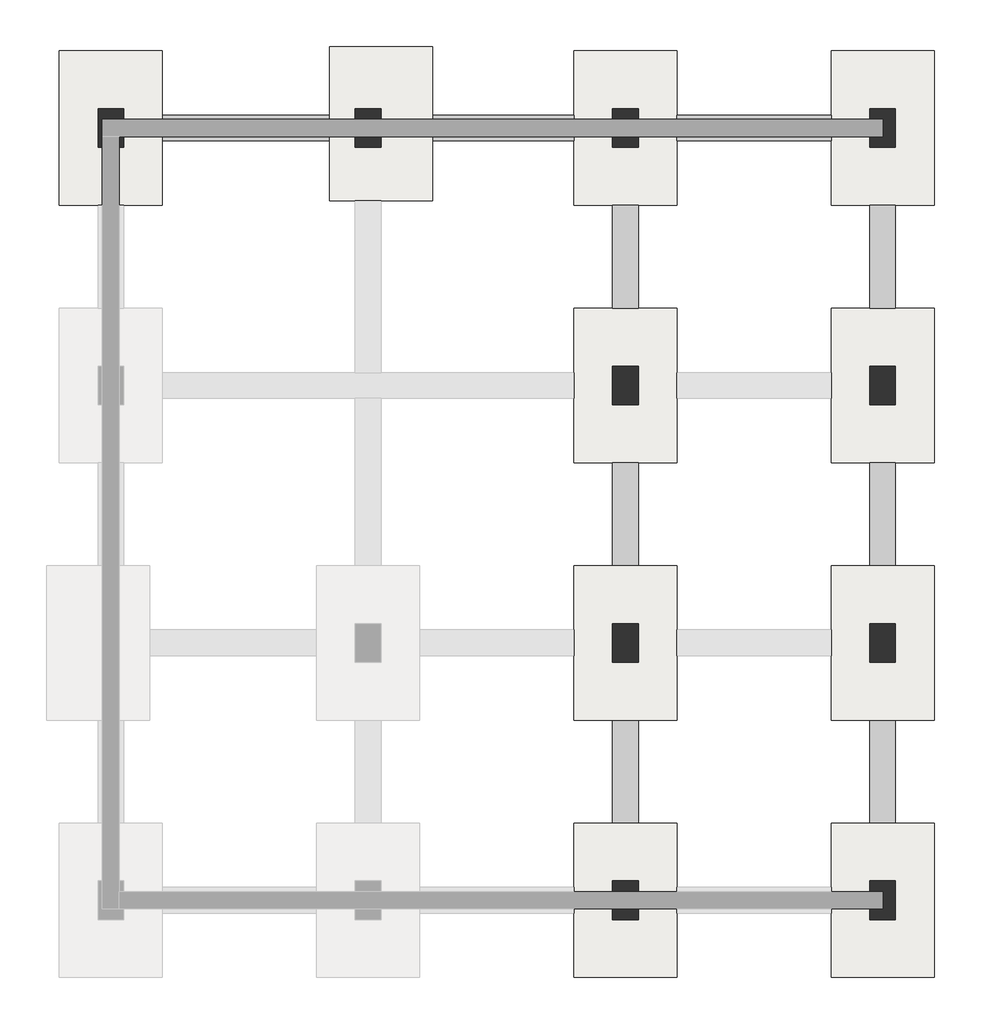
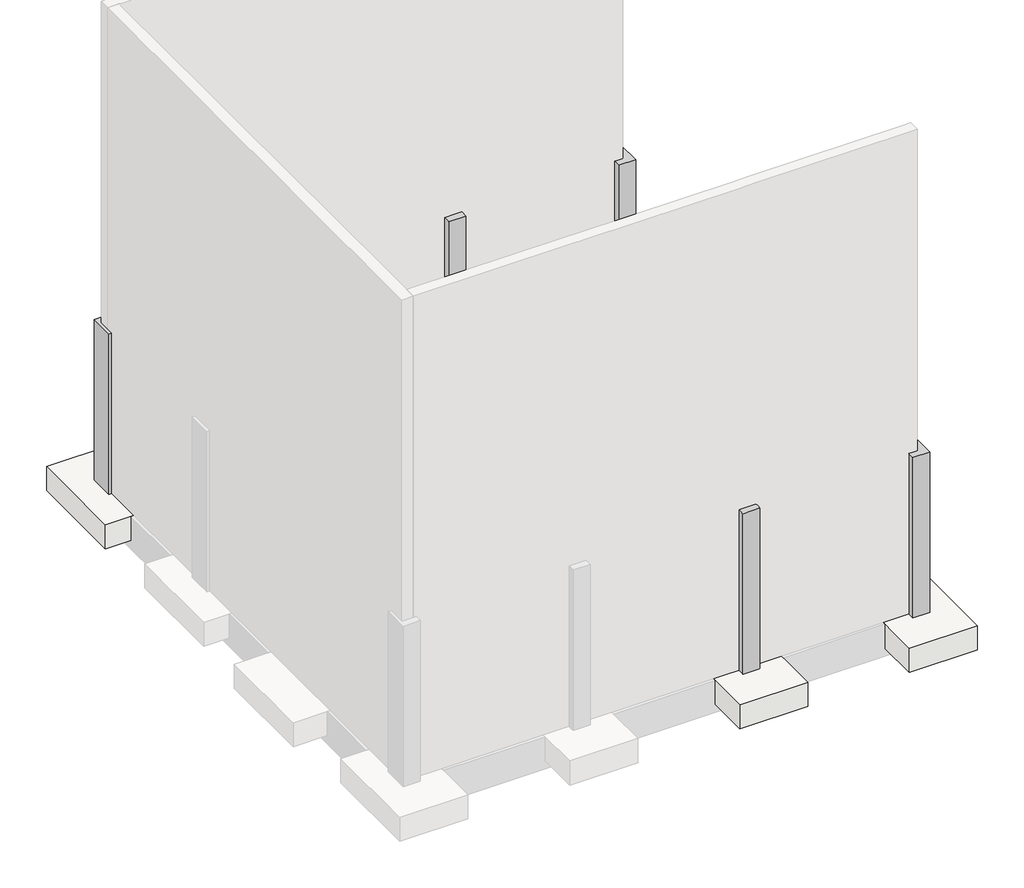
# One storey, part 2 of 2: 10 columns, 10 slabs, 3 beams.
"""IFC4 building model written with IfcOpenShell, lengths in millimetres."""

from ifc_helpers import new_model, si_unit, frame, origin, origin_with_axes, place, context, project, spatial, polyline, outline, extrude, faceted_brep, element, save

model = new_model("IFC4")

# Units and contexts
model_context = context("Model", 3, world=origin())
ifc_project = project(units=[si_unit("LENGTHUNIT", "METRE", prefix="MILLI")], contexts=[model_context])

# Site, building, storey
site = spatial("IfcSite", under=ifc_project)
building = spatial("IfcBuilding", under=site)
storey = spatial("IfcBuildingStorey", under=building, Elevation=0.0)

# Beams
placement = place(None, origin())
element("IfcBeam", 1, ObjectType="Concrete-Rectangular Beam : 12 x 24", at=placement, inside=storey, context=model_context, shape_type="Brep", body=[
    faceted_brep([(-15136.5609662, 12775.9972109, 0.0), (-15136.5609662, 12471.1972109, 0.0), (-13307.7609662, 12471.1972109, 0.0), (-13307.7609662, 12775.9972109, 0.0), (-21232.5609662, 12471.1972109, -457.2), (-21689.7609662, 12471.1972109, -457.2), (-21994.5609662, 12471.1972109, -457.2), (-21994.5609662, 12471.1972109, -609.6), (-21689.7609662, 12471.1972109, -609.6), (-18946.5609662, 12471.1972109, -609.6), (-18641.7609662, 12471.1972109, -609.6), (-15898.5609662, 12471.1972109, -609.6), (-15593.7609662, 12471.1972109, -609.6), (-12850.5609662, 12471.1972109, -609.6), (-12850.5609662, 12471.1972109, -457.2), (-13307.7609662, 12471.1972109, -457.2), (-15136.5609662, 12471.1972109, -457.2), (-15593.7609662, 12471.1972109, -457.2), (-15898.5609662, 12471.1972109, -457.2), (-16355.7609662, 12471.1972109, -457.2), (-16355.7609662, 12471.1972109, 0.0), (-18032.1609662, 12471.1972109, 0.0), (-18032.1609662, 12471.1972109, -457.2), (-18641.7609662, 12471.1972109, -457.2), (-18946.5609662, 12471.1972109, -457.2), (-19251.3609662, 12471.1972109, -457.2), (-19251.3609662, 12471.1972109, 0.0), (-21232.5609662, 12471.1972109, 0.0), (-21994.5609662, 12775.9972109, -609.6), (-12545.7609662, 12775.9972109, -609.6), (-12545.7609662, 12725.1972109, -609.6), (-12850.5609662, 12725.1972109, -609.6), (-21994.5609662, 12775.9972109, -457.2), (-21232.5609662, 12775.9972109, -457.2), (-21232.5609662, 12775.9972109, 0.0), (-19251.3609662, 12775.9972109, 0.0), (-19251.3609662, 12775.9972109, -457.2), (-18032.1609662, 12775.9972109, -457.2), (-18032.1609662, 12775.9972109, 0.0), (-16355.7609662, 12775.9972109, 0.0), (-16355.7609662, 12775.9972109, -457.2), (-15136.5609662, 12775.9972109, -457.2), (-13307.7609662, 12775.9972109, -457.2), (-12545.7609662, 12775.9972109, -457.2), (-12850.5609662, 12725.1972109, -457.2), (-12545.7609662, 12725.1972109, -457.2)], [[[0, 1, 2, 3]], [[4, 5, 6, 7, 8, 9, 10, 11, 12, 13, 14, 15, 2, 1, 16, 17, 18, 19, 20, 21, 22, 23, 24, 25, 26, 27]], [[7, 28, 29, 30, 31, 13, 12, 11, 10, 9, 8]], [[32, 33, 34, 35, 36, 37, 38, 39, 40, 41, 0, 3, 42, 43, 29, 28]], [[4, 33, 32, 6, 5]], [[33, 4, 27, 34]], [[22, 37, 36, 25, 24, 23]], [[37, 22, 21, 38]], [[25, 36, 35, 26]], [[34, 27, 26, 35]], [[16, 41, 40, 19, 18, 17]], [[41, 16, 1, 0]], [[19, 40, 39, 20]], [[42, 15, 14, 44, 45, 43]], [[15, 42, 3, 2]], [[28, 7, 6, 32]], [[29, 43, 45, 30]], [[38, 21, 20, 39]], [[31, 44, 14, 13]], [[44, 31, 30, 45]]]),
])
element("IfcBeam", 2, ObjectType="Concrete-Rectangular Beam : 12 x 24", at=placement, inside=storey, context=model_context, shape_type="Brep", body=[
    faceted_brep([(-12545.7609662, 5613.1972109, 0.0), (-12850.5609662, 5613.1972109, 0.0), (-12850.5609662, 4393.9972109, 0.0), (-12545.7609662, 4393.9972109, 0.0), (-12850.5609662, 11709.1972109, -457.2), (-12850.5609662, 12471.1972109, -457.2), (-12850.5609662, 12725.1972109, -457.2), (-12850.5609662, 12725.1972109, -609.6), (-12850.5609662, 12471.1972109, -609.6), (-12850.5609662, 9727.9972109, -609.6), (-12850.5609662, 9423.1972109, -609.6), (-12850.5609662, 6679.9972109, -609.6), (-12850.5609662, 6375.1972109, -609.6), (-12850.5609662, 3631.9972109, -609.6), (-12850.5609662, 3377.9972109, -609.6), (-12850.5609662, 3377.9972109, -457.2), (-12850.5609662, 3631.9972109, -457.2), (-12850.5609662, 4393.9972109, -457.2), (-12850.5609662, 5613.1972109, -457.2), (-12850.5609662, 6375.1972109, -457.2), (-12850.5609662, 6679.9972109, -457.2), (-12850.5609662, 7441.9972109, -457.2), (-12850.5609662, 7441.9972109, 0.0), (-12850.5609662, 8661.1972109, 0.0), (-12850.5609662, 8661.1972109, -457.2), (-12850.5609662, 9423.1972109, -457.2), (-12850.5609662, 9727.9972109, -457.2), (-12850.5609662, 10489.9972109, -457.2), (-12850.5609662, 10489.9972109, 0.0), (-12850.5609662, 11709.1972109, 0.0), (-12545.7609662, 12725.1972109, -609.6), (-12545.7609662, 3377.9972109, -609.6), (-12698.1609662, 3377.9972109, -609.6), (-12545.7609662, 12725.1972109, -457.2), (-12545.7609662, 11709.1972109, -457.2), (-12545.7609662, 11709.1972109, 0.0), (-12545.7609662, 10489.9972109, 0.0), (-12545.7609662, 10489.9972109, -457.2), (-12545.7609662, 8661.1972109, -457.2), (-12545.7609662, 8661.1972109, 0.0), (-12545.7609662, 7441.9972109, 0.0), (-12545.7609662, 7441.9972109, -457.2), (-12545.7609662, 5613.1972109, -457.2), (-12545.7609662, 4393.9972109, -457.2), (-12545.7609662, 3377.9972109, -457.2), (-12698.1609662, 3377.9972109, -457.2)], [[[0, 1, 2, 3]], [[4, 5, 6, 7, 8, 9, 10, 11, 12, 13, 14, 15, 16, 17, 2, 1, 18, 19, 20, 21, 22, 23, 24, 25, 26, 27, 28, 29]], [[7, 30, 31, 32, 14, 13, 12, 11, 10, 9, 8]], [[33, 34, 35, 36, 37, 38, 39, 40, 41, 42, 0, 3, 43, 44, 31, 30]], [[4, 34, 33, 6, 5]], [[34, 4, 29, 35]], [[24, 38, 37, 27, 26, 25]], [[38, 24, 23, 39]], [[27, 37, 36, 28]], [[35, 29, 28, 36]], [[18, 42, 41, 21, 20, 19]], [[42, 18, 1, 0]], [[21, 41, 40, 22]], [[39, 23, 22, 40]], [[43, 17, 16, 15, 45, 44]], [[17, 43, 3, 2]], [[30, 7, 6, 33]], [[14, 32, 31, 44, 45, 15]]]),
])
element("IfcBeam", 3, ObjectType="Concrete-Rectangular Beam : 12 x 24", at=placement, inside=storey, context=model_context, shape_type="SweptSolid", body=[
    extrude(outline(polyline([(5613.1972109, 0.0), (5613.1972109, -457.2), (6375.1972109, -457.2), (6375.1972109, -609.6), (3631.9972109, -609.6), (3631.9972109, -457.2), (4393.9972109, -457.2), (4393.9972109, 0.0), (5613.1972109, 0.0)])), frame((-15898.5609662, 0.0, 0.0), z_axis=(1.0, 0.0, 0.0), x_axis=(0.0, 1.0, 0.0)), (0.0, 0.0, 1.0), 304.8),
    extrude(outline(polyline([(12471.1972109, -457.2), (12471.1972109, -609.6), (9727.9972109, -609.6), (9727.9972109, -457.2), (10489.9972109, -457.2), (10489.9972109, 0.0), (11709.1972109, 0.0), (11709.1972109, -457.2), (12471.1972109, -457.2)])), frame((-15898.5609662, 0.0, 0.0), z_axis=(1.0, 0.0, 0.0), x_axis=(0.0, 1.0, 0.0)), (0.0, 0.0, 1.0), 304.8),
    extrude(outline(polyline([(8661.1972109, 0.0), (8661.1972109, -457.2), (9423.1972109, -457.2), (9423.1972109, -609.6), (6679.9972109, -609.6), (6679.9972109, -457.2), (7441.9972109, -457.2), (7441.9972109, 0.0), (8661.1972109, 0.0)])), frame((-15898.5609662, 0.0, 0.0), z_axis=(1.0, 0.0, 0.0), x_axis=(0.0, 1.0, 0.0)), (0.0, 0.0, 1.0), 304.8),
])

# Columns
element("IfcColumn", 4, ObjectType="Concrete-Rectangular-Column : 12 x 18", at=placement, inside=storey, context=model_context, shape_type="Brep", body=[
    faceted_brep([(-21689.7609662, 12521.9972109, 0.0), (-21689.7609662, 12394.9972109, 0.0), (-21740.5609662, 12394.9972109, 0.0), (-21740.5609662, 12521.9972109, 0.0), (-21689.7609662, 12394.9972109, 3048.0), (-21689.7609662, 12521.9972109, 3048.0), (-21740.5609662, 12394.9972109, 3048.0), (-21740.5609662, 12521.9972109, 3048.0)], [[[0, 1, 2, 3]], [[4, 1, 0, 5]], [[1, 4, 6, 2]], [[5, 0, 3, 7]], [[3, 2, 6, 7]], [[4, 5, 7, 6]]]),
    faceted_brep([(-21994.5609662, 12852.1972109, 0.0), (-21994.5609662, 12394.9972109, 0.0), (-21994.5609662, 12394.9972109, 3048.0), (-21994.5609662, 12852.1972109, 3048.0), (-21689.7609662, 12852.1972109, 0.0), (-21689.7609662, 12852.1972109, 3048.0), (-21943.7609662, 12394.9972109, 3048.0), (-21943.7609662, 12725.1972109, 3048.0), (-21689.7609662, 12725.1972109, 3048.0), (-21943.7609662, 12725.1972109, 0.0), (-21689.7609662, 12725.1972109, 0.0), (-21943.7609662, 12394.9972109, 0.0), (-21943.7609662, 12521.9972109, 0.0)], [[[0, 1, 2, 3]], [[4, 0, 3, 5]], [[3, 2, 6, 7, 8, 5]], [[9, 10, 8, 7]], [[4, 5, 8, 10]], [[9, 7, 6, 11, 12]], [[1, 0, 4, 10, 9, 12, 11]], [[2, 1, 11, 6]]]),
])
element("IfcColumn", 5, ObjectType="Concrete-Rectangular-Column : 12 x 18", at=placement, inside=storey, context=model_context, shape_type="Brep", body=[
    faceted_brep([(-18641.7609662, 12394.9972109, 0.0), (-18946.5609662, 12394.9972109, 0.0), (-18946.5609662, 12521.9972109, 0.0), (-18641.7609662, 12521.9972109, 0.0), (-18641.7609662, 12394.9972109, 3048.0), (-18641.7609662, 12521.9972109, 2438.4), (-18641.7609662, 12521.9972109, 2895.6), (-18641.7609662, 12521.9972109, 3048.0), (-18946.5609662, 12394.9972109, 3048.0), (-18946.5609662, 12521.9972109, 2438.4), (-18946.5609662, 12521.9972109, 2895.6), (-18946.5609662, 12521.9972109, 3048.0)], [[[0, 1, 2, 3]], [[4, 0, 3, 5, 6, 7]], [[1, 0, 4, 8]], [[3, 2, 9, 10, 11, 7, 6, 5]], [[1, 8, 11, 10, 9, 2]], [[8, 4, 7, 11]]]),
    faceted_brep([(-18946.5609662, 12852.1972109, 3048.0), (-18946.5609662, 12852.1972109, 0.0), (-18946.5609662, 12725.1972109, 0.0), (-18946.5609662, 12725.1972109, 2438.4), (-18946.5609662, 12725.1972109, 3048.0), (-18946.5609662, 12775.9972109, 3048.0), (-18641.7609662, 12852.1972109, 0.0), (-18641.7609662, 12852.1972109, 3048.0), (-18641.7609662, 12725.1972109, 3048.0), (-18641.7609662, 12775.9972109, 3048.0), (-18641.7609662, 12725.1972109, 0.0), (-18641.7609662, 12725.1972109, 2438.4)], [[[0, 1, 2, 3, 4, 5]], [[6, 1, 0, 7]], [[7, 0, 5, 4, 8, 9]], [[2, 10, 11, 8, 4, 3]], [[1, 6, 10, 2]], [[6, 7, 9, 8, 11, 10]]]),
])
element("IfcColumn", 6, ObjectType="Concrete-Rectangular-Column : 12 x 18", at=placement, inside=storey, context=model_context, shape_type="Brep", body=[
    faceted_brep([(-15593.7609662, 12394.9972109, 0.0), (-15898.5609662, 12394.9972109, 0.0), (-15898.5609662, 12521.9972109, 0.0), (-15593.7609662, 12521.9972109, 0.0), (-15593.7609662, 12394.9972109, 3048.0), (-15593.7609662, 12521.9972109, 2438.4), (-15593.7609662, 12521.9972109, 2895.6), (-15593.7609662, 12521.9972109, 3048.0), (-15898.5609662, 12394.9972109, 3048.0), (-15898.5609662, 12521.9972109, 2438.4), (-15898.5609662, 12521.9972109, 2895.6), (-15898.5609662, 12521.9972109, 3048.0)], [[[0, 1, 2, 3]], [[4, 0, 3, 5, 6, 7]], [[1, 0, 4, 8]], [[3, 2, 9, 10, 11, 7, 6, 5]], [[1, 8, 11, 10, 9, 2]], [[8, 4, 7, 11]]]),
    faceted_brep([(-15898.5609662, 12852.1972109, 3048.0), (-15898.5609662, 12852.1972109, 0.0), (-15898.5609662, 12725.1972109, 0.0), (-15898.5609662, 12725.1972109, 2438.4), (-15898.5609662, 12725.1972109, 3048.0), (-15898.5609662, 12775.9972109, 3048.0), (-15593.7609662, 12852.1972109, 0.0), (-15593.7609662, 12852.1972109, 3048.0), (-15593.7609662, 12725.1972109, 3048.0), (-15593.7609662, 12775.9972109, 3048.0), (-15593.7609662, 12725.1972109, 0.0), (-15593.7609662, 12725.1972109, 2438.4)], [[[0, 1, 2, 3, 4, 5]], [[6, 1, 0, 7]], [[7, 0, 5, 4, 8, 9]], [[2, 10, 11, 8, 4, 3]], [[1, 6, 10, 2]], [[6, 7, 9, 8, 11, 10]]]),
])
element("IfcColumn", 7, ObjectType="Concrete-Rectangular-Column : 12 x 18", at=placement, inside=storey, context=model_context, shape_type="Brep", body=[
    faceted_brep([(-15898.5609662, 9346.9972109, 0.0), (-15898.5609662, 9804.1972109, 0.0), (-15593.7609662, 9804.1972109, 0.0), (-15593.7609662, 9346.9972109, 0.0), (-15898.5609662, 9346.9972109, 3048.0), (-15898.5609662, 9804.1972109, 3048.0), (-15898.5609662, 9804.1972109, 2895.6), (-15898.5609662, 9804.1972109, 2438.4), (-15898.5609662, 9346.9972109, 2438.4), (-15898.5609662, 9346.9972109, 2895.6), (-15593.7609662, 9804.1972109, 3048.0), (-15593.7609662, 9804.1972109, 2895.6), (-15593.7609662, 9804.1972109, 2438.4), (-15593.7609662, 9346.9972109, 3048.0), (-15593.7609662, 9346.9972109, 2895.6), (-15593.7609662, 9346.9972109, 2438.4)], [[[0, 1, 2, 3]], [[4, 5, 6, 7, 1, 0, 8, 9]], [[5, 10, 11, 12, 2, 1, 7, 6]], [[10, 13, 14, 15, 3, 2, 12, 11]], [[13, 4, 9, 8, 0, 3, 15, 14]], [[4, 13, 10, 5]]]),
])
element("IfcColumn", 8, ObjectType="Concrete-Rectangular-Column : 12 x 18", at=placement, inside=storey, context=model_context, shape_type="Brep", body=[
    faceted_brep([(-15898.5609662, 6298.9972109, 0.0), (-15898.5609662, 6756.1972109, 0.0), (-15593.7609662, 6756.1972109, 0.0), (-15593.7609662, 6298.9972109, 0.0), (-15898.5609662, 6298.9972109, 3048.0), (-15898.5609662, 6756.1972109, 3048.0), (-15898.5609662, 6756.1972109, 2895.6), (-15898.5609662, 6756.1972109, 2438.4), (-15898.5609662, 6298.9972109, 2438.4), (-15898.5609662, 6298.9972109, 2895.6), (-15593.7609662, 6756.1972109, 3048.0), (-15593.7609662, 6756.1972109, 2895.6), (-15593.7609662, 6756.1972109, 2438.4), (-15593.7609662, 6298.9972109, 3048.0), (-15593.7609662, 6298.9972109, 2895.6), (-15593.7609662, 6298.9972109, 2438.4)], [[[0, 1, 2, 3]], [[4, 5, 6, 7, 1, 0, 8, 9]], [[5, 10, 11, 12, 2, 1, 7, 6]], [[10, 13, 14, 15, 3, 2, 12, 11]], [[13, 4, 9, 8, 0, 3, 15, 14]], [[4, 13, 10, 5]]]),
])
element("IfcColumn", 9, ObjectType="Concrete-Rectangular-Column : 12 x 18", at=placement, inside=storey, context=model_context, shape_type="Brep", body=[
    faceted_brep([(-15593.7609662, 3250.9972109, 0.0), (-15898.5609662, 3250.9972109, 0.0), (-15898.5609662, 3377.9972109, 0.0), (-15593.7609662, 3377.9972109, 0.0), (-15593.7609662, 3250.9972109, 3048.0), (-15593.7609662, 3377.9972109, 2438.4), (-15593.7609662, 3377.9972109, 3048.0), (-15593.7609662, 3327.1972109, 3048.0), (-15898.5609662, 3250.9972109, 3048.0), (-15898.5609662, 3377.9972109, 2438.4), (-15898.5609662, 3377.9972109, 3048.0), (-15898.5609662, 3327.1972109, 3048.0)], [[[0, 1, 2, 3]], [[4, 0, 3, 5, 6, 7]], [[1, 0, 4, 8]], [[3, 2, 9, 10, 6, 5]], [[1, 8, 11, 10, 9, 2]], [[8, 4, 7, 6, 10, 11]]]),
    faceted_brep([(-15898.5609662, 3708.1972109, 3048.0), (-15898.5609662, 3708.1972109, 0.0), (-15898.5609662, 3581.1972109, 0.0), (-15898.5609662, 3581.1972109, 2438.4), (-15898.5609662, 3581.1972109, 2895.6), (-15898.5609662, 3581.1972109, 3048.0), (-15593.7609662, 3708.1972109, 0.0), (-15593.7609662, 3708.1972109, 3048.0), (-15593.7609662, 3581.1972109, 3048.0), (-15593.7609662, 3581.1972109, 0.0), (-15593.7609662, 3581.1972109, 2438.4), (-15593.7609662, 3581.1972109, 2895.6)], [[[0, 1, 2, 3, 4, 5]], [[6, 1, 0, 7]], [[7, 0, 5, 8]], [[2, 9, 10, 11, 8, 5, 4, 3]], [[1, 6, 9, 2]], [[6, 7, 8, 11, 10, 9]]]),
])
element("IfcColumn", 10, ObjectType="Concrete-Rectangular-Column : 12 x 18", at=placement, inside=storey, context=model_context, shape_type="SweptSolid", body=[
    extrude(outline(polyline([(-12850.5609662, 12852.1972109), (-12545.7609662, 12852.1972109), (-12545.7609662, 12394.9972109), (-12850.5609662, 12394.9972109), (-12850.5609662, 12521.9972109), (-12698.1609662, 12521.9972109), (-12698.1609662, 12725.1972109), (-12850.5609662, 12725.1972109), (-12850.5609662, 12852.1972109)])), origin_with_axes(), (0.0, 0.0, 1.0), 3048.0),
])
element("IfcColumn", 11, ObjectType="Concrete-Rectangular-Column : 12 x 18", at=placement, inside=storey, context=model_context, shape_type="Brep", body=[
    faceted_brep([(-12850.5609662, 9346.9972109, 0.0), (-12850.5609662, 9804.1972109, 0.0), (-12545.7609662, 9804.1972109, 0.0), (-12545.7609662, 9346.9972109, 0.0), (-12850.5609662, 9346.9972109, 3048.0), (-12850.5609662, 9804.1972109, 3048.0), (-12850.5609662, 9804.1972109, 2895.6), (-12850.5609662, 9804.1972109, 2438.4), (-12850.5609662, 9346.9972109, 2438.4), (-12850.5609662, 9346.9972109, 2895.6), (-12698.1609662, 9804.1972109, 3048.0), (-12545.7609662, 9804.1972109, 3048.0), (-12545.7609662, 9804.1972109, 2438.4), (-12545.7609662, 9346.9972109, 3048.0), (-12545.7609662, 9346.9972109, 2438.4), (-12698.1609662, 9346.9972109, 3048.0)], [[[0, 1, 2, 3]], [[4, 5, 6, 7, 1, 0, 8, 9]], [[5, 10, 11, 12, 2, 1, 7, 6]], [[11, 13, 14, 3, 2, 12]], [[13, 15, 4, 9, 8, 0, 3, 14]], [[4, 15, 13, 11, 10, 5]]]),
])
element("IfcColumn", 12, ObjectType="Concrete-Rectangular-Column : 12 x 18", at=placement, inside=storey, context=model_context, shape_type="Brep", body=[
    faceted_brep([(-12850.5609662, 6298.9972109, 0.0), (-12850.5609662, 6756.1972109, 0.0), (-12545.7609662, 6756.1972109, 0.0), (-12545.7609662, 6298.9972109, 0.0), (-12850.5609662, 6298.9972109, 3048.0), (-12850.5609662, 6756.1972109, 3048.0), (-12850.5609662, 6756.1972109, 2895.6), (-12850.5609662, 6756.1972109, 2438.4), (-12850.5609662, 6298.9972109, 2438.4), (-12850.5609662, 6298.9972109, 2895.6), (-12698.1609662, 6756.1972109, 3048.0), (-12545.7609662, 6756.1972109, 3048.0), (-12545.7609662, 6756.1972109, 2438.4), (-12545.7609662, 6298.9972109, 3048.0), (-12545.7609662, 6298.9972109, 2438.4), (-12698.1609662, 6298.9972109, 3048.0)], [[[0, 1, 2, 3]], [[4, 5, 6, 7, 1, 0, 8, 9]], [[5, 10, 11, 12, 2, 1, 7, 6]], [[11, 13, 14, 3, 2, 12]], [[13, 15, 4, 9, 8, 0, 3, 14]], [[4, 15, 13, 11, 10, 5]]]),
])
element("IfcColumn", 13, ObjectType="Concrete-Rectangular-Column : 12 x 18", at=placement, inside=storey, context=model_context, shape_type="SweptSolid", body=[
    extrude(outline(polyline([(-12850.5609662, 3708.1972109), (-12545.7609662, 3708.1972109), (-12545.7609662, 3250.9972109), (-12850.5609662, 3250.9972109), (-12850.5609662, 3377.9972109), (-12698.1609662, 3377.9972109), (-12698.1609662, 3581.1972109), (-12850.5609662, 3581.1972109), (-12850.5609662, 3708.1972109)])), origin_with_axes(), (0.0, 0.0, 1.0), 3048.0),
])

# Slabs
element("IfcSlab", 14, ObjectType="Footing-Rectangular : 72\" x 48\" x 18\"", at=placement, inside=storey, context=model_context, shape_type="Brep", body=[
    faceted_brep([(-22451.7609662, 11709.1972109, 0.0), (-21994.5609662, 11709.1972109, 0.0), (-21689.7609662, 11709.1972109, 0.0), (-21232.5609662, 11709.1972109, 0.0), (-21232.5609662, 12471.1972109, 0.0), (-21232.5609662, 12775.9972109, 0.0), (-21232.5609662, 13537.9972109, 0.0), (-22451.7609662, 13537.9972109, 0.0), (-22451.7609662, 11709.1972109, -457.2), (-22451.7609662, 13537.9972109, -457.2), (-21232.5609662, 13537.9972109, -457.2), (-21232.5609662, 12775.9972109, -457.2), (-21232.5609662, 12471.1972109, -457.2), (-21232.5609662, 11709.1972109, -457.2), (-21689.7609662, 11709.1972109, -457.2), (-21994.5609662, 11709.1972109, -457.2)], [[[0, 1, 2, 3, 4, 5, 6, 7]], [[8, 9, 10, 11, 12, 13, 14, 15]], [[3, 2, 1, 0, 8, 15, 14, 13]], [[6, 5, 4, 3, 13, 12, 11, 10]], [[7, 6, 10, 9]], [[0, 7, 9, 8]]]),
])
element("IfcSlab", 15, ObjectType="Footing-Rectangular : 72\" x 48\" x 18\"", at=placement, inside=storey, context=model_context, shape_type="Brep", body=[
    faceted_brep([(-19251.3609662, 11759.9972109, 0.0), (-18946.5609662, 11759.9972109, 0.0), (-18641.7609662, 11759.9972109, 0.0), (-18032.1609662, 11759.9972109, 0.0), (-18032.1609662, 12471.1972109, 0.0), (-18032.1609662, 12775.9972109, 0.0), (-18032.1609662, 13588.7972109, 0.0), (-19251.3609662, 13588.7972109, 0.0), (-19251.3609662, 12775.9972109, 0.0), (-19251.3609662, 12471.1972109, 0.0), (-19251.3609662, 11759.9972109, -457.2), (-19251.3609662, 12471.1972109, -457.2), (-19251.3609662, 12775.9972109, -457.2), (-19251.3609662, 13588.7972109, -457.2), (-18032.1609662, 13588.7972109, -457.2), (-18032.1609662, 12775.9972109, -457.2), (-18032.1609662, 12471.1972109, -457.2), (-18032.1609662, 11759.9972109, -457.2), (-18641.7609662, 11759.9972109, -457.2), (-18946.5609662, 11759.9972109, -457.2)], [[[0, 1, 2, 3, 4, 5, 6, 7, 8, 9]], [[10, 11, 12, 13, 14, 15, 16, 17, 18, 19]], [[3, 2, 1, 0, 10, 19, 18, 17]], [[6, 5, 4, 3, 17, 16, 15, 14]], [[7, 6, 14, 13]], [[0, 9, 8, 7, 13, 12, 11, 10]]]),
])
element("IfcSlab", 16, ObjectType="Footing-Rectangular : 72\" x 48\" x 18\"", at=placement, inside=storey, context=model_context, shape_type="Brep", body=[
    faceted_brep([(-16355.7609662, 11709.1972109, 0.0), (-15898.5609662, 11709.1972109, 0.0), (-15593.7609662, 11709.1972109, 0.0), (-15136.5609662, 11709.1972109, 0.0), (-15136.5609662, 12471.1972109, 0.0), (-15136.5609662, 12775.9972109, 0.0), (-15136.5609662, 13537.9972109, 0.0), (-16355.7609662, 13537.9972109, 0.0), (-16355.7609662, 12775.9972109, 0.0), (-16355.7609662, 12471.1972109, 0.0), (-16355.7609662, 11709.1972109, -457.2), (-16355.7609662, 12471.1972109, -457.2), (-16355.7609662, 12775.9972109, -457.2), (-16355.7609662, 13537.9972109, -457.2), (-15136.5609662, 13537.9972109, -457.2), (-15136.5609662, 12775.9972109, -457.2), (-15136.5609662, 12471.1972109, -457.2), (-15136.5609662, 11709.1972109, -457.2), (-15593.7609662, 11709.1972109, -457.2), (-15898.5609662, 11709.1972109, -457.2)], [[[0, 1, 2, 3, 4, 5, 6, 7, 8, 9]], [[10, 11, 12, 13, 14, 15, 16, 17, 18, 19]], [[3, 2, 1, 0, 10, 19, 18, 17]], [[6, 5, 4, 3, 17, 16, 15, 14]], [[7, 6, 14, 13]], [[0, 9, 8, 7, 13, 12, 11, 10]]]),
])
element("IfcSlab", 17, ObjectType="Footing-Rectangular : 72\" x 48\" x 18\"", at=placement, inside=storey, context=model_context, shape_type="Brep", body=[
    faceted_brep([(-16355.7609662, 8661.1972109, 0.0), (-15898.5609662, 8661.1972109, 0.0), (-15593.7609662, 8661.1972109, 0.0), (-15136.5609662, 8661.1972109, 0.0), (-15136.5609662, 9423.1972109, 0.0), (-15136.5609662, 9727.9972109, 0.0), (-15136.5609662, 10489.9972109, 0.0), (-15593.7609662, 10489.9972109, 0.0), (-15898.5609662, 10489.9972109, 0.0), (-16355.7609662, 10489.9972109, 0.0), (-16355.7609662, 9727.9972109, 0.0), (-16355.7609662, 9423.1972109, 0.0), (-16355.7609662, 8661.1972109, -457.2), (-16355.7609662, 9423.1972109, -457.2), (-16355.7609662, 9727.9972109, -457.2), (-16355.7609662, 10489.9972109, -457.2), (-15898.5609662, 10489.9972109, -457.2), (-15593.7609662, 10489.9972109, -457.2), (-15136.5609662, 10489.9972109, -457.2), (-15136.5609662, 9727.9972109, -457.2), (-15136.5609662, 9423.1972109, -457.2), (-15136.5609662, 8661.1972109, -457.2), (-15593.7609662, 8661.1972109, -457.2), (-15898.5609662, 8661.1972109, -457.2)], [[[0, 1, 2, 3, 4, 5, 6, 7, 8, 9, 10, 11]], [[12, 13, 14, 15, 16, 17, 18, 19, 20, 21, 22, 23]], [[3, 2, 1, 0, 12, 23, 22, 21]], [[6, 5, 4, 3, 21, 20, 19, 18]], [[9, 8, 7, 6, 18, 17, 16, 15]], [[0, 11, 10, 9, 15, 14, 13, 12]]]),
])
element("IfcSlab", 18, ObjectType="Footing-Rectangular : 72\" x 48\" x 18\"", at=placement, inside=storey, context=model_context, shape_type="Brep", body=[
    faceted_brep([(-16355.7609662, 5613.1972109, 0.0), (-15898.5609662, 5613.1972109, 0.0), (-15593.7609662, 5613.1972109, 0.0), (-15136.5609662, 5613.1972109, 0.0), (-15136.5609662, 6375.1972109, 0.0), (-15136.5609662, 6679.9972109, 0.0), (-15136.5609662, 7441.9972109, 0.0), (-15593.7609662, 7441.9972109, 0.0), (-15898.5609662, 7441.9972109, 0.0), (-16355.7609662, 7441.9972109, 0.0), (-16355.7609662, 6679.9972109, 0.0), (-16355.7609662, 6375.1972109, 0.0), (-16355.7609662, 5613.1972109, -457.2), (-16355.7609662, 6375.1972109, -457.2), (-16355.7609662, 6679.9972109, -457.2), (-16355.7609662, 7441.9972109, -457.2), (-15898.5609662, 7441.9972109, -457.2), (-15593.7609662, 7441.9972109, -457.2), (-15136.5609662, 7441.9972109, -457.2), (-15136.5609662, 6679.9972109, -457.2), (-15136.5609662, 6375.1972109, -457.2), (-15136.5609662, 5613.1972109, -457.2), (-15593.7609662, 5613.1972109, -457.2), (-15898.5609662, 5613.1972109, -457.2)], [[[0, 1, 2, 3, 4, 5, 6, 7, 8, 9, 10, 11]], [[12, 13, 14, 15, 16, 17, 18, 19, 20, 21, 22, 23]], [[3, 2, 1, 0, 12, 23, 22, 21]], [[6, 5, 4, 3, 21, 20, 19, 18]], [[9, 8, 7, 6, 18, 17, 16, 15]], [[0, 11, 10, 9, 15, 14, 13, 12]]]),
])
element("IfcSlab", 19, ObjectType="Footing-Rectangular : 72\" x 48\" x 18\"", at=placement, inside=storey, context=model_context, shape_type="Brep", body=[
    faceted_brep([(-16355.7609662, 2565.1972109, 0.0), (-15136.5609662, 2565.1972109, 0.0), (-15136.5609662, 3327.1972109, 0.0), (-15136.5609662, 3631.9972109, 0.0), (-15136.5609662, 4393.9972109, 0.0), (-15593.7609662, 4393.9972109, 0.0), (-15898.5609662, 4393.9972109, 0.0), (-16355.7609662, 4393.9972109, 0.0), (-16355.7609662, 3631.9972109, 0.0), (-16355.7609662, 3327.1972109, 0.0), (-16355.7609662, 2565.1972109, -457.2), (-16355.7609662, 3327.1972109, -457.2), (-16355.7609662, 3631.9972109, -457.2), (-16355.7609662, 4393.9972109, -457.2), (-15898.5609662, 4393.9972109, -457.2), (-15593.7609662, 4393.9972109, -457.2), (-15136.5609662, 4393.9972109, -457.2), (-15136.5609662, 3631.9972109, -457.2), (-15136.5609662, 3327.1972109, -457.2), (-15136.5609662, 2565.1972109, -457.2)], [[[0, 1, 2, 3, 4, 5, 6, 7, 8, 9]], [[10, 11, 12, 13, 14, 15, 16, 17, 18, 19]], [[1, 0, 10, 19]], [[4, 3, 2, 1, 19, 18, 17, 16]], [[7, 6, 5, 4, 16, 15, 14, 13]], [[0, 9, 8, 7, 13, 12, 11, 10]]]),
])
element("IfcSlab", 20, ObjectType="Footing-Rectangular : 72\" x 48\" x 18\"", at=placement, inside=storey, context=model_context, shape_type="Brep", body=[
    faceted_brep([(-13307.7609662, 11709.1972109, 0.0), (-12850.5609662, 11709.1972109, 0.0), (-12545.7609662, 11709.1972109, 0.0), (-12088.5609662, 11709.1972109, 0.0), (-12088.5609662, 13537.9972109, 0.0), (-13307.7609662, 13537.9972109, 0.0), (-13307.7609662, 12775.9972109, 0.0), (-13307.7609662, 12471.1972109, 0.0), (-13307.7609662, 11709.1972109, -457.2), (-13307.7609662, 12471.1972109, -457.2), (-13307.7609662, 12775.9972109, -457.2), (-13307.7609662, 13537.9972109, -457.2), (-12088.5609662, 13537.9972109, -457.2), (-12088.5609662, 11709.1972109, -457.2), (-12545.7609662, 11709.1972109, -457.2), (-12850.5609662, 11709.1972109, -457.2)], [[[0, 1, 2, 3, 4, 5, 6, 7]], [[8, 9, 10, 11, 12, 13, 14, 15]], [[3, 2, 1, 0, 8, 15, 14, 13]], [[4, 3, 13, 12]], [[5, 4, 12, 11]], [[0, 7, 6, 5, 11, 10, 9, 8]]]),
])
element("IfcSlab", 21, ObjectType="Footing-Rectangular : 72\" x 48\" x 18\"", at=placement, inside=storey, context=model_context, shape_type="Brep", body=[
    faceted_brep([(-13307.7609662, 8661.1972109, 0.0), (-12850.5609662, 8661.1972109, 0.0), (-12545.7609662, 8661.1972109, 0.0), (-12088.5609662, 8661.1972109, 0.0), (-12088.5609662, 10489.9972109, 0.0), (-12545.7609662, 10489.9972109, 0.0), (-12850.5609662, 10489.9972109, 0.0), (-13307.7609662, 10489.9972109, 0.0), (-13307.7609662, 9727.9972109, 0.0), (-13307.7609662, 9423.1972109, 0.0), (-13307.7609662, 8661.1972109, -457.2), (-13307.7609662, 9423.1972109, -457.2), (-13307.7609662, 9727.9972109, -457.2), (-13307.7609662, 10489.9972109, -457.2), (-12850.5609662, 10489.9972109, -457.2), (-12545.7609662, 10489.9972109, -457.2), (-12088.5609662, 10489.9972109, -457.2), (-12088.5609662, 8661.1972109, -457.2), (-12545.7609662, 8661.1972109, -457.2), (-12850.5609662, 8661.1972109, -457.2)], [[[0, 1, 2, 3, 4, 5, 6, 7, 8, 9]], [[10, 11, 12, 13, 14, 15, 16, 17, 18, 19]], [[3, 2, 1, 0, 10, 19, 18, 17]], [[4, 3, 17, 16]], [[7, 6, 5, 4, 16, 15, 14, 13]], [[0, 9, 8, 7, 13, 12, 11, 10]]]),
])
element("IfcSlab", 22, ObjectType="Footing-Rectangular : 72\" x 48\" x 18\"", at=placement, inside=storey, context=model_context, shape_type="Brep", body=[
    faceted_brep([(-13307.7609662, 5613.1972109, 0.0), (-12850.5609662, 5613.1972109, 0.0), (-12545.7609662, 5613.1972109, 0.0), (-12088.5609662, 5613.1972109, 0.0), (-12088.5609662, 7441.9972109, 0.0), (-12545.7609662, 7441.9972109, 0.0), (-12850.5609662, 7441.9972109, 0.0), (-13307.7609662, 7441.9972109, 0.0), (-13307.7609662, 6679.9972109, 0.0), (-13307.7609662, 6375.1972109, 0.0), (-13307.7609662, 5613.1972109, -457.2), (-13307.7609662, 6375.1972109, -457.2), (-13307.7609662, 6679.9972109, -457.2), (-13307.7609662, 7441.9972109, -457.2), (-12850.5609662, 7441.9972109, -457.2), (-12545.7609662, 7441.9972109, -457.2), (-12088.5609662, 7441.9972109, -457.2), (-12088.5609662, 5613.1972109, -457.2), (-12545.7609662, 5613.1972109, -457.2), (-12850.5609662, 5613.1972109, -457.2)], [[[0, 1, 2, 3, 4, 5, 6, 7, 8, 9]], [[10, 11, 12, 13, 14, 15, 16, 17, 18, 19]], [[3, 2, 1, 0, 10, 19, 18, 17]], [[4, 3, 17, 16]], [[7, 6, 5, 4, 16, 15, 14, 13]], [[0, 9, 8, 7, 13, 12, 11, 10]]]),
])
element("IfcSlab", 23, ObjectType="Footing-Rectangular : 72\" x 48\" x 18\"", at=placement, inside=storey, context=model_context, shape_type="Brep", body=[
    faceted_brep([(-13307.7609662, 2565.1972109, 0.0), (-12088.5609662, 2565.1972109, 0.0), (-12088.5609662, 4393.9972109, 0.0), (-12545.7609662, 4393.9972109, 0.0), (-12850.5609662, 4393.9972109, 0.0), (-13307.7609662, 4393.9972109, 0.0), (-13307.7609662, 3631.9972109, 0.0), (-13307.7609662, 3327.1972109, 0.0), (-13307.7609662, 2565.1972109, -457.2), (-13307.7609662, 3327.1972109, -457.2), (-13307.7609662, 3631.9972109, -457.2), (-13307.7609662, 4393.9972109, -457.2), (-12850.5609662, 4393.9972109, -457.2), (-12545.7609662, 4393.9972109, -457.2), (-12088.5609662, 4393.9972109, -457.2), (-12088.5609662, 2565.1972109, -457.2)], [[[0, 1, 2, 3, 4, 5, 6, 7]], [[8, 9, 10, 11, 12, 13, 14, 15]], [[1, 0, 8, 15]], [[2, 1, 15, 14]], [[5, 4, 3, 2, 14, 13, 12, 11]], [[0, 7, 6, 5, 11, 10, 9, 8]]]),
])

save(model, "model.ifc")

# Revit data of these elements
# Type "Concrete-Rectangular Beam : 12 x 24"
#   Assembly Code = "B10"
#   Length [instance default] = 5' - 0"
#   b = 1' - 0"
#   h = 2' - 0"
#   Structural Material [instance default] = Concrete, Cast-in-Place gray
# Type "Concrete-Rectangular-Column : 12 x 18"
#   Assembly Code = "B10"
#   b = 1' - 0"
#   h = 1' - 6"
#   Structural Material [instance default] = Concrete, Cast-in-Place gray
# Type "Footing-Rectangular : 72\" x 48\" x 18\""
#   Assembly Code = "A1010100"
#   Width = 4' - 0"
#   Length = 6' - 0"
#   Foundation Thickness = 1' - 6"
#   Structural Material [instance default] = Concrete, Cast-in-Place gray
# Elements 1, 2, 3 (IfcBeam, "Concrete-Rectangular Beam : 12 x 24")
#   Structural Material = Concrete, Cast-in-Place gray
#   Phase Created = New Construction
#   Materials on its faces: "Concrete, Cast-in-Place gray"
# Elements 4, 5, 6, 7, 8, 9, 10, 11, 12, 13 (IfcColumn, "Concrete-Rectangular-Column : 12 x 18")
#   Comments = ""
#   Structural Material = Concrete, Cast-in-Place gray
#   Phase Created = New Construction
#   Materials on its faces: "Concrete, Cast-in-Place gray"
# Elements 14, 15, 16, 17, 18, 19, 20, 21, 22, 23 (IfcSlab, "Footing-Rectangular : 72\" x 48\" x 18\"")
#   Structural Material = Concrete, Cast-in-Place gray
#   Phase Created = New Construction
#   Materials on its faces: "Concrete, Cast-in-Place gray"
# Materials
#   "Concrete, Cast-in-Place gray": class "Concrete", colour RGB 192 192 192, transparency 0, Description = "Cast-in-place concrete", Cost = 0
